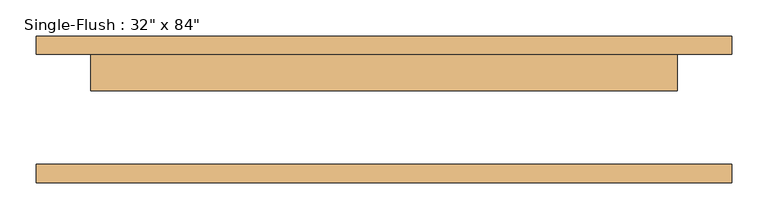
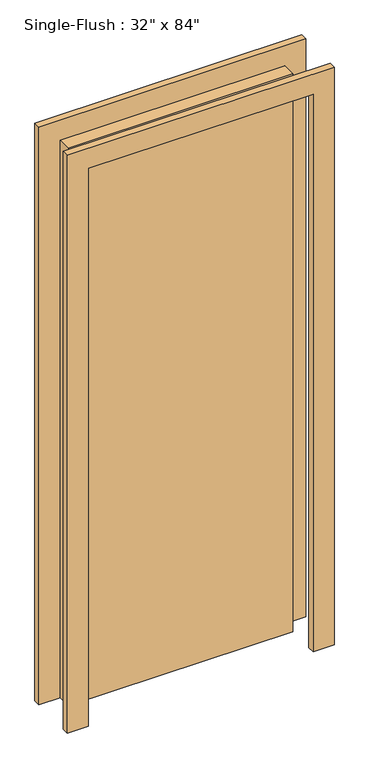
"""IFC4 building model written with IfcOpenShell, lengths in millimetres: door geometry."""

from ifc_helpers import new_model, si_unit, frame, origin, origin_with_axes, place, context, project, spatial, polyline, outline, extrude, source, transform, mapped, element, save


def door_377e7377(model_context):
    return source(origin(), model_context, "Body", "SweptSolid", [
        extrude(outline(polyline([(2209.8, -482.6), (0.0, -482.6), (0.0, -406.4), (2133.6, -406.4), (2133.6, 406.4), (0.0, 406.4), (0.0, 482.6), (2209.8, 482.6), (2209.8, -482.6)])), frame((0.0, 76.2, 0.0), z_axis=(0.0, 1.0, 0.0), x_axis=(0.0, 0.0, 1.0)), (0.0, 0.0, 1.0), 25.4),
        extrude(outline(polyline([(2209.8, 482.6), (2209.8, -482.6), (0.0, -482.6), (0.0, -406.4), (2133.6, -406.4), (2133.6, 406.4), (0.0, 406.4), (0.0, 482.6), (2209.8, 482.6)])), frame((0.0, -101.6, 0.0), z_axis=(0.0, 1.0, 0.0), x_axis=(0.0, 0.0, 1.0)), (0.0, 0.0, 1.0), 25.4),
        extrude(outline(polyline([(406.4, 25.4), (-406.4, 25.4), (-406.4, 76.2), (406.4, 76.2), (406.4, 25.4)])), origin_with_axes(), (0.0, 0.0, 1.0), 2133.6),
    ])


if __name__ == "__main__":
    model = new_model("IFC4")
    model_context = context("Model", 3, world=origin())
    ifc_project = project(units=[si_unit("LENGTHUNIT", "METRE", prefix="MILLI")], contexts=[model_context])
    site = spatial("IfcSite", under=ifc_project)
    building = spatial("IfcBuilding", under=site)
    placement = place(None, origin())
    door_shape = door_377e7377(model_context)
    element("IfcDoor", 1, ObjectType="Single-Flush : 32\" x 84\"", at=placement, inside=building, context=model_context, shape_type="MappedRepresentation", body=[
        mapped(door_shape, transform((0.0, 0.0, 0.0), x_axis=(1.0, 0.0, 0.0), y_axis=(0.0, 1.0, 0.0), z_axis=(0.0, 0.0, 1.0))),
    ])
    save(model, "model.ifc")

# Revit data of these elements
# Type "Single-Flush : 32\" x 84\""
#   Type Mark = "3"
#   Construction Type Id = "MDOOR"
#   Assembly Code = "C1020"
#   Analytic Construction = "Metal"
#   Thickness = 0' - 2"
#   Heat Transfer Coefficient (U) = 0.651978 BTU/(h·ft²·°F)
#   Height = 7' - 0"
#   Trim Projection Ext = 0' - 1"
#   Trim Projection Int = 0' - 1"
#   Trim Width = 0' - 3"
#   Width = 2' - 8"
#   Define Thermal Properties by = 1
#   Define Thermal Properties by = 1
#   Door Material = Door - Panel
#   Frame Material = Door - Frame
#   Visual Light Transmittance = 0
#   Solar Heat Gain Coefficient = 0
#   Function = (empty or 0)
#   Wall Closure = (empty or 0)
# Element 1 (IfcDoor, "Single-Flush : 32\" x 84\"")
#   Materials on its faces: "Door - Frame", "Door - Panel"
# Materials
#   "Door - Panel": class "Wood", colour RGB 210 159 95, transparency 0, Cost = 0
#   "Door - Frame": colour RGB 118 70 51, transparency 0, Cost = 0
